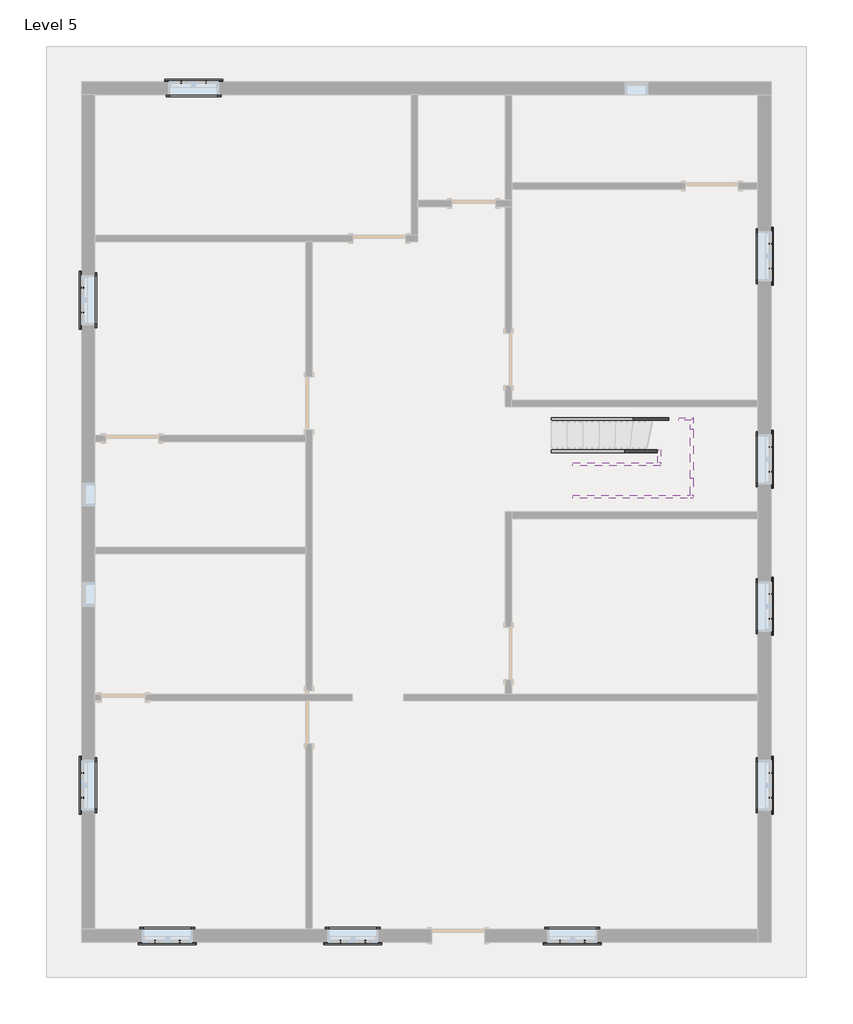
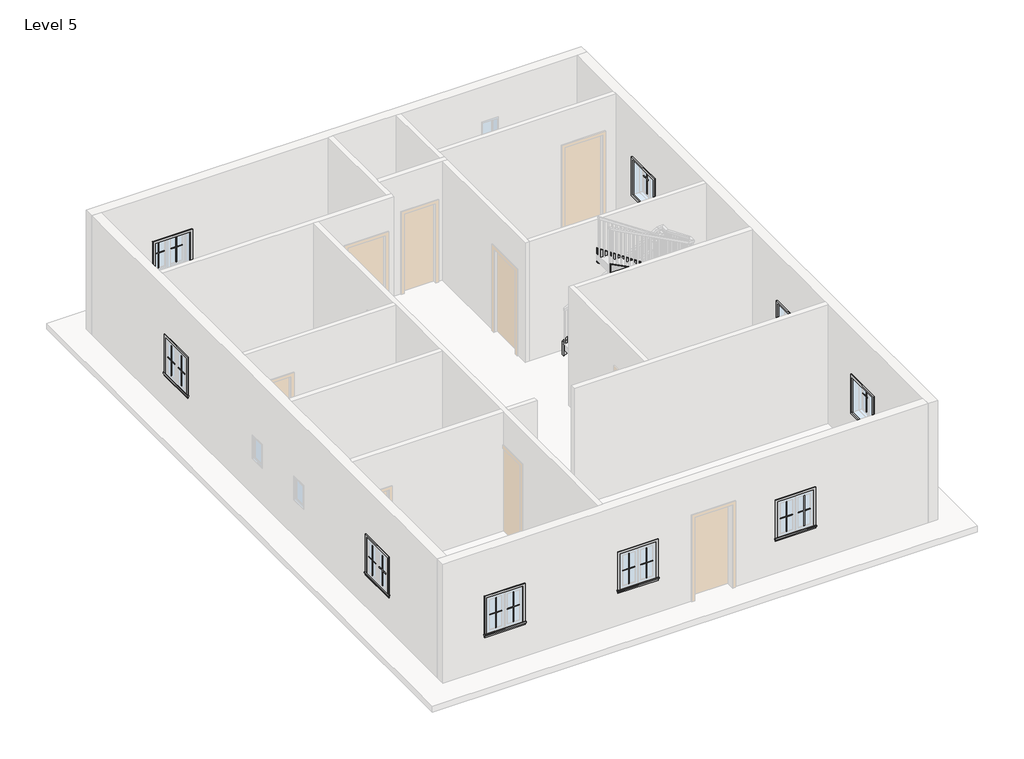
# One storey, part 3 of 3: 40 proxies, 9 members.
"""IFC4 building model written with IfcOpenShell, lengths in millimetres."""

from ifc_helpers import new_model, si_unit, frame, origin, place, context, project, spatial, polyline, outline, extrude, transform, mapped, element, save
from components import muntin_pattern_2x2_muntin_pattern_2x2_b3fe6957, muntin_pattern_2x2_muntin_pattern_2x2_3e0ecaf2, trim_window_exterior_flat_with_sill_41619996, trim_window_interior_flat_picture_frame_51c85655

model = new_model("IFC4")

# Units and contexts
model_context = context("Model", 3, world=origin())
ifc_project = project(units=[si_unit("LENGTHUNIT", "METRE", prefix="MILLI")], contexts=[model_context])

# Site, building, storey
site = spatial("IfcSite", under=ifc_project)
building = spatial("IfcBuilding", under=site)
storey = spatial("IfcBuildingStorey", under=building, Name="Level 5", Elevation=9601.2)

# Proxies
placement = place(None, origin())
muntin_pattern_2x2_muntin_pattern_2x2_shape = muntin_pattern_2x2_muntin_pattern_2x2_b3fe6957(model_context)
element("IfcBuildingElementProxy", 1, Name="Muntin Pattern_2x2 : Muntin Pattern_2x2", ObjectType="Muntin Pattern_2x2 : Muntin Pattern_2x2", at=placement, inside=storey, context=model_context, shape_type="MappedRepresentation", body=[
    mapped(muntin_pattern_2x2_muntin_pattern_2x2_shape, transform((-5581.2368007, 9072.452558, 10585.45), x_axis=(1.0, 0.0, 0.0), y_axis=(0.0, 1.0, 0.0), z_axis=(0.0, 0.0, 1.0))),
])
element("IfcBuildingElementProxy", 2, Name="Muntin Pattern_2x2 : Muntin Pattern_2x2", ObjectType="Muntin Pattern_2x2 : Muntin Pattern_2x2", at=placement, inside=storey, context=model_context, shape_type="MappedRepresentation", body=[
    mapped(muntin_pattern_2x2_muntin_pattern_2x2_shape, transform((-7300.4993007, 5076.715058, 10585.45), x_axis=(0.0, 1.0, 0.0), y_axis=(-1.0, 0.0, 0.0), z_axis=(0.0, 0.0, 1.0))),
])
element("IfcBuildingElementProxy", 3, Name="Muntin Pattern_2x2 : Muntin Pattern_2x2", ObjectType="Muntin Pattern_2x2 : Muntin Pattern_2x2", at=placement, inside=storey, context=model_context, shape_type="MappedRepresentation", body=[
    mapped(muntin_pattern_2x2_muntin_pattern_2x2_shape, transform((4643.8506993, 6267.340058, 10585.45), x_axis=(0.0, -1.0, 0.0), y_axis=(1.0, 0.0, 0.0), z_axis=(0.0, 0.0, 1.0))),
])
element("IfcBuildingElementProxy", 4, Name="Muntin Pattern_2x2 : Muntin Pattern_2x2", ObjectType="Muntin Pattern_2x2 : Muntin Pattern_2x2", at=placement, inside=storey, context=model_context, shape_type="MappedRepresentation", body=[
    mapped(muntin_pattern_2x2_muntin_pattern_2x2_shape, transform((4643.8506993, 2743.090058, 10585.45), x_axis=(0.0, -1.0, 0.0), y_axis=(1.0, 0.0, 0.0), z_axis=(0.0, 0.0, 1.0))),
])
element("IfcBuildingElementProxy", 5, Name="Muntin Pattern_2x2 : Muntin Pattern_2x2", ObjectType="Muntin Pattern_2x2 : Muntin Pattern_2x2", at=placement, inside=storey, context=model_context, shape_type="MappedRepresentation", body=[
    mapped(muntin_pattern_2x2_muntin_pattern_2x2_shape, transform((4643.8506993, 190.390058, 10585.45), x_axis=(0.0, -1.0, 0.0), y_axis=(1.0, 0.0, 0.0), z_axis=(0.0, 0.0, 1.0))),
])
element("IfcBuildingElementProxy", 6, Name="Muntin Pattern_2x2 : Muntin Pattern_2x2", ObjectType="Muntin Pattern_2x2 : Muntin Pattern_2x2", at=placement, inside=storey, context=model_context, shape_type="MappedRepresentation", body=[
    mapped(muntin_pattern_2x2_muntin_pattern_2x2_shape, transform((4643.8506993, -2914.759942, 10585.45), x_axis=(0.0, -1.0, 0.0), y_axis=(1.0, 0.0, 0.0), z_axis=(0.0, 0.0, 1.0))),
])
element("IfcBuildingElementProxy", 7, Name="Muntin Pattern_2x2 : Muntin Pattern_2x2", ObjectType="Muntin Pattern_2x2 : Muntin Pattern_2x2", at=placement, inside=storey, context=model_context, shape_type="MappedRepresentation", body=[
    mapped(muntin_pattern_2x2_muntin_pattern_2x2_shape, transform((1419.6381993, -5843.697442, 10585.45), x_axis=(-1.0, 0.0, 0.0), y_axis=(0.0, -1.0, 0.0), z_axis=(0.0, 0.0, 1.0))),
])
element("IfcBuildingElementProxy", 8, Name="Muntin Pattern_2x2 : Muntin Pattern_2x2", ObjectType="Muntin Pattern_2x2 : Muntin Pattern_2x2", at=placement, inside=storey, context=model_context, shape_type="MappedRepresentation", body=[
    mapped(muntin_pattern_2x2_muntin_pattern_2x2_shape, transform((-2390.3618007, -5843.697442, 10585.45), x_axis=(-1.0, 0.0, 0.0), y_axis=(0.0, -1.0, 0.0), z_axis=(0.0, 0.0, 1.0))),
])
element("IfcBuildingElementProxy", 9, Name="Muntin Pattern_2x2 : Muntin Pattern_2x2", ObjectType="Muntin Pattern_2x2 : Muntin Pattern_2x2", at=placement, inside=storey, context=model_context, shape_type="MappedRepresentation", body=[
    mapped(muntin_pattern_2x2_muntin_pattern_2x2_shape, transform((-5609.8118007, -5843.697442, 10585.45), x_axis=(-1.0, 0.0, 0.0), y_axis=(0.0, -1.0, 0.0), z_axis=(0.0, 0.0, 1.0))),
])
element("IfcBuildingElementProxy", 10, Name="Muntin Pattern_2x2 : Muntin Pattern_2x2", ObjectType="Muntin Pattern_2x2 : Muntin Pattern_2x2", at=placement, inside=storey, context=model_context, shape_type="MappedRepresentation", body=[
    mapped(muntin_pattern_2x2_muntin_pattern_2x2_shape, transform((-7300.4993007, -3343.384942, 10585.45), x_axis=(0.0, 1.0, 0.0), y_axis=(-1.0, 0.0, 0.0), z_axis=(0.0, 0.0, 1.0))),
])
muntin_pattern_2x2_muntin_pattern_2x2_2_shape = muntin_pattern_2x2_muntin_pattern_2x2_3e0ecaf2(model_context)
element("IfcBuildingElementProxy", 11, Name="Muntin Pattern_2x2 : Muntin Pattern_2x2", ObjectType="Muntin Pattern_2x2 : Muntin Pattern_2x2", at=placement, inside=storey, context=model_context, shape_type="MappedRepresentation", body=[
    mapped(muntin_pattern_2x2_muntin_pattern_2x2_2_shape, transform((-5152.6118007, 9072.452558, 10585.45), x_axis=(-1.0, 0.0, 0.0), y_axis=(0.0, -1.0, 0.0), z_axis=(0.0, 0.0, 1.0))),
])
element("IfcBuildingElementProxy", 12, Name="Muntin Pattern_2x2 : Muntin Pattern_2x2", ObjectType="Muntin Pattern_2x2 : Muntin Pattern_2x2", at=placement, inside=storey, context=model_context, shape_type="MappedRepresentation", body=[
    mapped(muntin_pattern_2x2_muntin_pattern_2x2_2_shape, transform((-7300.4993007, 5505.340058, 10585.45), x_axis=(0.0, -1.0, 0.0), y_axis=(1.0, 0.0, 0.0), z_axis=(0.0, 0.0, 1.0))),
])
element("IfcBuildingElementProxy", 13, Name="Muntin Pattern_2x2 : Muntin Pattern_2x2", ObjectType="Muntin Pattern_2x2 : Muntin Pattern_2x2", at=placement, inside=storey, context=model_context, shape_type="MappedRepresentation", body=[
    mapped(muntin_pattern_2x2_muntin_pattern_2x2_2_shape, transform((4643.8506993, 5838.715058, 10585.45), x_axis=(0.0, 1.0, 0.0), y_axis=(-1.0, 0.0, 0.0), z_axis=(0.0, 0.0, 1.0))),
])
element("IfcBuildingElementProxy", 14, Name="Muntin Pattern_2x2 : Muntin Pattern_2x2", ObjectType="Muntin Pattern_2x2 : Muntin Pattern_2x2", at=placement, inside=storey, context=model_context, shape_type="MappedRepresentation", body=[
    mapped(muntin_pattern_2x2_muntin_pattern_2x2_2_shape, transform((4643.8506993, 2314.465058, 10585.45), x_axis=(0.0, 1.0, 0.0), y_axis=(-1.0, 0.0, 0.0), z_axis=(0.0, 0.0, 1.0))),
])
element("IfcBuildingElementProxy", 15, Name="Muntin Pattern_2x2 : Muntin Pattern_2x2", ObjectType="Muntin Pattern_2x2 : Muntin Pattern_2x2", at=placement, inside=storey, context=model_context, shape_type="MappedRepresentation", body=[
    mapped(muntin_pattern_2x2_muntin_pattern_2x2_2_shape, transform((4643.8506993, -238.234942, 10585.45), x_axis=(0.0, 1.0, 0.0), y_axis=(-1.0, 0.0, 0.0), z_axis=(0.0, 0.0, 1.0))),
])
element("IfcBuildingElementProxy", 16, Name="Muntin Pattern_2x2 : Muntin Pattern_2x2", ObjectType="Muntin Pattern_2x2 : Muntin Pattern_2x2", at=placement, inside=storey, context=model_context, shape_type="MappedRepresentation", body=[
    mapped(muntin_pattern_2x2_muntin_pattern_2x2_2_shape, transform((4643.8506993, -3343.384942, 10585.45), x_axis=(0.0, 1.0, 0.0), y_axis=(-1.0, 0.0, 0.0), z_axis=(0.0, 0.0, 1.0))),
])
element("IfcBuildingElementProxy", 17, Name="Muntin Pattern_2x2 : Muntin Pattern_2x2", ObjectType="Muntin Pattern_2x2 : Muntin Pattern_2x2", at=placement, inside=storey, context=model_context, shape_type="MappedRepresentation", body=[
    mapped(muntin_pattern_2x2_muntin_pattern_2x2_2_shape, transform((991.0131993, -5843.697442, 10585.45), x_axis=(1.0, 0.0, 0.0), y_axis=(0.0, 1.0, 0.0), z_axis=(0.0, 0.0, 1.0))),
])
element("IfcBuildingElementProxy", 18, Name="Muntin Pattern_2x2 : Muntin Pattern_2x2", ObjectType="Muntin Pattern_2x2 : Muntin Pattern_2x2", at=placement, inside=storey, context=model_context, shape_type="MappedRepresentation", body=[
    mapped(muntin_pattern_2x2_muntin_pattern_2x2_2_shape, transform((-2818.9868007, -5843.697442, 10585.45), x_axis=(1.0, 0.0, 0.0), y_axis=(0.0, 1.0, 0.0), z_axis=(0.0, 0.0, 1.0))),
])
element("IfcBuildingElementProxy", 19, Name="Muntin Pattern_2x2 : Muntin Pattern_2x2", ObjectType="Muntin Pattern_2x2 : Muntin Pattern_2x2", at=placement, inside=storey, context=model_context, shape_type="MappedRepresentation", body=[
    mapped(muntin_pattern_2x2_muntin_pattern_2x2_2_shape, transform((-6038.4368007, -5843.697442, 10585.45), x_axis=(1.0, 0.0, 0.0), y_axis=(0.0, 1.0, 0.0), z_axis=(0.0, 0.0, 1.0))),
])
element("IfcBuildingElementProxy", 20, Name="Muntin Pattern_2x2 : Muntin Pattern_2x2", ObjectType="Muntin Pattern_2x2 : Muntin Pattern_2x2", at=placement, inside=storey, context=model_context, shape_type="MappedRepresentation", body=[
    mapped(muntin_pattern_2x2_muntin_pattern_2x2_2_shape, transform((-7300.4993007, -2914.759942, 10585.45), x_axis=(0.0, -1.0, 0.0), y_axis=(1.0, 0.0, 0.0), z_axis=(0.0, 0.0, 1.0))),
])
trim_window_exterior_flat_with_sill_shape = trim_window_exterior_flat_with_sill_41619996(model_context)
element("IfcBuildingElementProxy", 21, Name="Trim-Window-Exterior-Flat : with Sill", ObjectType="Trim-Window-Exterior-Flat : with Sill", at=placement, inside=storey, context=model_context, shape_type="MappedRepresentation", body=[
    mapped(trim_window_exterior_flat_with_sill_shape, transform((-5366.9243007, 9081.977558, 11430.0), x_axis=(-1.0, 0.0, 0.0), y_axis=(0.0, 0.0, 1.0), z_axis=(0.0, 1.0, 0.0))),
])
element("IfcBuildingElementProxy", 22, Name="Trim-Window-Exterior-Flat : with Sill", ObjectType="Trim-Window-Exterior-Flat : with Sill", at=placement, inside=storey, context=model_context, shape_type="MappedRepresentation", body=[
    mapped(trim_window_exterior_flat_with_sill_shape, transform((-7310.0243007, 5291.027558, 11430.0), x_axis=(0.0, -1.0, 0.0), y_axis=(0.0, 0.0, 1.0), z_axis=(-1.0, 0.0, 0.0))),
])
element("IfcBuildingElementProxy", 23, Name="Trim-Window-Exterior-Flat : with Sill", ObjectType="Trim-Window-Exterior-Flat : with Sill", at=placement, inside=storey, context=model_context, shape_type="MappedRepresentation", body=[
    mapped(trim_window_exterior_flat_with_sill_shape, transform((4653.3756993, 6053.027558, 11430.0), x_axis=(0.0, 1.0, 0.0), y_axis=(0.0, 0.0, 1.0), z_axis=(1.0, 0.0, 0.0))),
])
element("IfcBuildingElementProxy", 24, Name="Trim-Window-Exterior-Flat : with Sill", ObjectType="Trim-Window-Exterior-Flat : with Sill", at=placement, inside=storey, context=model_context, shape_type="MappedRepresentation", body=[
    mapped(trim_window_exterior_flat_with_sill_shape, transform((4653.3756993, 2528.777558, 11430.0), x_axis=(0.0, 1.0, 0.0), y_axis=(0.0, 0.0, 1.0), z_axis=(1.0, 0.0, 0.0))),
])
element("IfcBuildingElementProxy", 25, Name="Trim-Window-Exterior-Flat : with Sill", ObjectType="Trim-Window-Exterior-Flat : with Sill", at=placement, inside=storey, context=model_context, shape_type="MappedRepresentation", body=[
    mapped(trim_window_exterior_flat_with_sill_shape, transform((4653.3756993, -23.922442, 11430.0), x_axis=(0.0, 1.0, 0.0), y_axis=(0.0, 0.0, 1.0), z_axis=(1.0, 0.0, 0.0))),
])
element("IfcBuildingElementProxy", 26, Name="Trim-Window-Exterior-Flat : with Sill", ObjectType="Trim-Window-Exterior-Flat : with Sill", at=placement, inside=storey, context=model_context, shape_type="MappedRepresentation", body=[
    mapped(trim_window_exterior_flat_with_sill_shape, transform((4653.3756993, -3129.072442, 11430.0), x_axis=(0.0, 1.0, 0.0), y_axis=(0.0, 0.0, 1.0), z_axis=(1.0, 0.0, 0.0))),
])
element("IfcBuildingElementProxy", 27, Name="Trim-Window-Exterior-Flat : with Sill", ObjectType="Trim-Window-Exterior-Flat : with Sill", at=placement, inside=storey, context=model_context, shape_type="MappedRepresentation", body=[
    mapped(trim_window_exterior_flat_with_sill_shape, transform((1205.3256993, -5853.222442, 11430.0), x_axis=(1.0, 0.0, 0.0), y_axis=(0.0, 0.0, 1.0), z_axis=(0.0, -1.0, 0.0))),
])
element("IfcBuildingElementProxy", 28, Name="Trim-Window-Exterior-Flat : with Sill", ObjectType="Trim-Window-Exterior-Flat : with Sill", at=placement, inside=storey, context=model_context, shape_type="MappedRepresentation", body=[
    mapped(trim_window_exterior_flat_with_sill_shape, transform((-2604.6743007, -5853.222442, 11430.0), x_axis=(1.0, 0.0, 0.0), y_axis=(0.0, 0.0, 1.0), z_axis=(0.0, -1.0, 0.0))),
])
element("IfcBuildingElementProxy", 29, Name="Trim-Window-Exterior-Flat : with Sill", ObjectType="Trim-Window-Exterior-Flat : with Sill", at=placement, inside=storey, context=model_context, shape_type="MappedRepresentation", body=[
    mapped(trim_window_exterior_flat_with_sill_shape, transform((-5824.1243007, -5853.222442, 11430.0), x_axis=(1.0, 0.0, 0.0), y_axis=(0.0, 0.0, 1.0), z_axis=(0.0, -1.0, 0.0))),
])
element("IfcBuildingElementProxy", 30, Name="Trim-Window-Exterior-Flat : with Sill", ObjectType="Trim-Window-Exterior-Flat : with Sill", at=placement, inside=storey, context=model_context, shape_type="MappedRepresentation", body=[
    mapped(trim_window_exterior_flat_with_sill_shape, transform((-7310.0243007, -3129.072442, 11430.0), x_axis=(0.0, -1.0, 0.0), y_axis=(0.0, 0.0, 1.0), z_axis=(-1.0, 0.0, 0.0))),
])
trim_window_interior_flat_picture_frame_shape = trim_window_interior_flat_picture_frame_51c85655(model_context)
element("IfcBuildingElementProxy", 31, Name="Trim-Window-Interior-Flat : Picture Frame", ObjectType="Trim-Window-Interior-Flat : Picture Frame", at=placement, inside=storey, context=model_context, shape_type="MappedRepresentation", body=[
    mapped(trim_window_interior_flat_picture_frame_shape, transform((-5366.9243007, 8853.377558, 11430.0), x_axis=(1.0, 0.0, 0.0), y_axis=(0.0, 0.0, 1.0), z_axis=(0.0, -1.0, 0.0))),
])
element("IfcBuildingElementProxy", 32, Name="Trim-Window-Interior-Flat : Picture Frame", ObjectType="Trim-Window-Interior-Flat : Picture Frame", at=placement, inside=storey, context=model_context, shape_type="MappedRepresentation", body=[
    mapped(trim_window_interior_flat_picture_frame_shape, transform((-7081.4243007, 5291.027558, 11430.0), x_axis=(0.0, 1.0, 0.0), y_axis=(0.0, 0.0, 1.0), z_axis=(1.0, 0.0, 0.0))),
])
element("IfcBuildingElementProxy", 33, Name="Trim-Window-Interior-Flat : Picture Frame", ObjectType="Trim-Window-Interior-Flat : Picture Frame", at=placement, inside=storey, context=model_context, shape_type="MappedRepresentation", body=[
    mapped(trim_window_interior_flat_picture_frame_shape, transform((4424.7756993, 6053.027558, 11430.0), x_axis=(0.0, -1.0, 0.0), y_axis=(0.0, 0.0, 1.0), z_axis=(-1.0, 0.0, 0.0))),
])
element("IfcBuildingElementProxy", 34, Name="Trim-Window-Interior-Flat : Picture Frame", ObjectType="Trim-Window-Interior-Flat : Picture Frame", at=placement, inside=storey, context=model_context, shape_type="MappedRepresentation", body=[
    mapped(trim_window_interior_flat_picture_frame_shape, transform((4424.7756993, 2528.777558, 11430.0), x_axis=(0.0, -1.0, 0.0), y_axis=(0.0, 0.0, 1.0), z_axis=(-1.0, 0.0, 0.0))),
])
element("IfcBuildingElementProxy", 35, Name="Trim-Window-Interior-Flat : Picture Frame", ObjectType="Trim-Window-Interior-Flat : Picture Frame", at=placement, inside=storey, context=model_context, shape_type="MappedRepresentation", body=[
    mapped(trim_window_interior_flat_picture_frame_shape, transform((4424.7756993, -23.922442, 11430.0), x_axis=(0.0, -1.0, 0.0), y_axis=(0.0, 0.0, 1.0), z_axis=(-1.0, 0.0, 0.0))),
])
element("IfcBuildingElementProxy", 36, Name="Trim-Window-Interior-Flat : Picture Frame", ObjectType="Trim-Window-Interior-Flat : Picture Frame", at=placement, inside=storey, context=model_context, shape_type="MappedRepresentation", body=[
    mapped(trim_window_interior_flat_picture_frame_shape, transform((4424.7756993, -3129.072442, 11430.0), x_axis=(0.0, -1.0, 0.0), y_axis=(0.0, 0.0, 1.0), z_axis=(-1.0, 0.0, 0.0))),
])
element("IfcBuildingElementProxy", 37, Name="Trim-Window-Interior-Flat : Picture Frame", ObjectType="Trim-Window-Interior-Flat : Picture Frame", at=placement, inside=storey, context=model_context, shape_type="MappedRepresentation", body=[
    mapped(trim_window_interior_flat_picture_frame_shape, transform((1205.3256993, -5624.622442, 11430.0), x_axis=(-1.0, 0.0, 0.0), y_axis=(0.0, 0.0, 1.0), z_axis=(0.0, 1.0, 0.0))),
])
element("IfcBuildingElementProxy", 38, Name="Trim-Window-Interior-Flat : Picture Frame", ObjectType="Trim-Window-Interior-Flat : Picture Frame", at=placement, inside=storey, context=model_context, shape_type="MappedRepresentation", body=[
    mapped(trim_window_interior_flat_picture_frame_shape, transform((-2604.6743007, -5624.622442, 11430.0), x_axis=(-1.0, 0.0, 0.0), y_axis=(0.0, 0.0, 1.0), z_axis=(0.0, 1.0, 0.0))),
])
element("IfcBuildingElementProxy", 39, Name="Trim-Window-Interior-Flat : Picture Frame", ObjectType="Trim-Window-Interior-Flat : Picture Frame", at=placement, inside=storey, context=model_context, shape_type="MappedRepresentation", body=[
    mapped(trim_window_interior_flat_picture_frame_shape, transform((-5824.1243007, -5624.622442, 11430.0), x_axis=(-1.0, 0.0, 0.0), y_axis=(0.0, 0.0, 1.0), z_axis=(0.0, 1.0, 0.0))),
])
element("IfcBuildingElementProxy", 40, Name="Trim-Window-Interior-Flat : Picture Frame", ObjectType="Trim-Window-Interior-Flat : Picture Frame", at=placement, inside=storey, context=model_context, shape_type="MappedRepresentation", body=[
    mapped(trim_window_interior_flat_picture_frame_shape, transform((-7081.4243007, -3129.072442, 11430.0), x_axis=(0.0, 1.0, 0.0), y_axis=(0.0, 0.0, 1.0), z_axis=(1.0, 0.0, 0.0))),
])

# Members
element("IfcMember", 41, ObjectType="Stringer - 2\" Width", at=placement, inside=storey, context=model_context, shape_type="SweptSolid", body=[
    extrude(outline(polyline([(9989.6746569, 838.4202681), (9639.0072902, 838.4202681), (10898.6160324, 3052.6525996), (11249.2833991, 3052.6525996), (9989.6746569, 838.4202681)])), frame((0.0, 3202.4524989, 0.0), z_axis=(0.0, 1.0, 0.0), x_axis=(0.0, 0.0, 1.0)), (0.0, 0.0, 1.0), 50.8),
])
element("IfcMember", 42, ObjectType="Stringer - 2\" Width", at=placement, inside=storey, context=model_context, shape_type="SweptSolid", body=[
    extrude(outline(polyline([(3052.6525996, 3202.4524989), (3052.6525996, 3253.2524989), (3298.782332, 3253.2524989), (3247.982332, 3202.4524989), (3052.6525996, 3202.4524989)])), frame((0.0, 0.0, 10898.6160324), z_axis=(0.0, 0.0, 1.0), x_axis=(1.0, 0.0, 0.0)), (0.0, 0.0, 1.0), 350.6673667),
])
element("IfcMember", 43, ObjectType="Stringer - 2\" Width", at=placement, inside=storey, context=model_context, shape_type="SweptSolid", body=[
    extrude(outline(polyline([(3247.982332, 3202.4524989), (3298.782332, 3253.2524989), (3298.782332, 3048.1586437), (3247.982332, 3048.1586437), (3247.982332, 3202.4524989)])), frame((0.0, 0.0, 10898.6160324), z_axis=(0.0, 0.0, 1.0), x_axis=(1.0, 0.0, 0.0)), (0.0, 0.0, 1.0), 350.6673667),
])
element("IfcMember", 44, ObjectType="Stringer - 2\" Width", at=placement, inside=storey, context=model_context, shape_type="SweptSolid", body=[
    extrude(outline(polyline([(3048.1586437, 11249.2833991), (3048.1586437, 10898.6160324), (2198.376501, 11254.1779505), (2198.376501, 11604.8453172), (3048.1586437, 11249.2833991)])), frame((3247.982332, 0.0, 0.0), z_axis=(1.0, 0.0, 0.0), x_axis=(0.0, 1.0, 0.0)), (0.0, 0.0, 1.0), 50.8),
])
element("IfcMember", 45, ObjectType="Stringer - 2\" Width", at=placement, inside=storey, context=model_context, shape_type="SweptSolid", body=[
    extrude(outline(polyline([(3247.982332, 2198.376501), (3298.782332, 2198.376501), (3298.782332, 1905.9026171), (3247.982332, 1905.9026171), (3247.982332, 2198.376501)])), frame((0.0, 0.0, 11263.1761112), z_axis=(0.0, 0.0, 1.0), x_axis=(1.0, 0.0, 0.0)), (0.0, 0.0, 1.0), 330.4053693),
])
element("IfcMember", 46, ObjectType="Stringer - 2\" Width", at=placement, inside=storey, context=model_context, shape_type="SweptSolid", body=[
    extrude(outline(polyline([(9975.2558321, 838.4202681), (9612.3163437, 838.4202681), (10808.3401496, 2688.6073911), (11171.2796379, 2688.6073911), (9975.2558321, 838.4202681)])), frame((0.0, 2643.077558, 0.0), z_axis=(0.0, 1.0, 0.0), x_axis=(0.0, 0.0, 1.0)), (0.0, 0.0, 1.0), 50.8),
])
element("IfcMember", 47, ObjectType="Stringer - 2\" Width", at=placement, inside=storey, context=model_context, shape_type="SweptSolid", body=[
    extrude(outline(polyline([(2693.877558, 11338.6149577), (2693.877558, 10891.3996268), (2465.277558, 11136.8439445), (2465.277558, 11584.0592754), (2693.877558, 11338.6149577)])), frame((2688.6073911, 0.0, 0.0), z_axis=(1.0, 0.0, 0.0), x_axis=(0.0, 1.0, 0.0)), (0.0, 0.0, 1.0), 50.8),
])
element("IfcMember", 48, ObjectType="Stringer - 2\" Width", at=placement, inside=storey, context=model_context, shape_type="SweptSolid", body=[
    extrude(outline(polyline([(11301.9150039, 2739.4073911), (11671.891358, 2739.4073911), (12723.0229383, 1211.6756993), (12353.0465842, 1211.6756993), (11301.9150039, 2739.4073911)])), frame((0.0, 2414.477558, 0.0), z_axis=(0.0, 1.0, 0.0), x_axis=(0.0, 0.0, 1.0)), (0.0, 0.0, 1.0), 50.8),
])
element("IfcMember", 49, ObjectType="Stringer - 2\" Width", at=placement, inside=storey, context=model_context, shape_type="SweptSolid", body=[
    extrude(outline(polyline([(11288.7814805, 3298.782332), (11567.1410006, 3298.782332), (12653.442202, 1211.6756993), (12323.0368327, 1211.6756993), (11288.7814805, 3198.7868271), (11288.7814805, 3298.782332)])), frame((0.0, 1855.1026171, 0.0), z_axis=(0.0, 1.0, 0.0), x_axis=(0.0, 0.0, 1.0)), (0.0, 0.0, 1.0), 50.8),
])

save(model, "model.ifc")

# Revit data of these elements
# Type "Muntin Pattern_2x2 : Muntin Pattern_2x2"
#   Width [instance default] = 4' - 0"
#   Thickness = 0' - 0 1/2"
#   Height [instance default] = 4' - 0"
#   Distance = 0' - 0 3/4"
#   Interior Material [instance default] = none
#   Exterior Material [instance default] = none
#   Default Elevation = 0
# Type "Trim-Window-Exterior-Flat : with Sill"
#   Trim Width = 0' - 2 1/4"
#   Trim Thickness_Picture Frame = 0' - 1 1/4"
#   Trim Thickness_with Sill = 0' - 0 3/4"
#   Sill Thickness = 0' - 1 1/4"
#   Opening Width [instance default] = 2' - 0"
#   Opening Height [instance default] = 3' - 0"
#   Default Elevation = 4' - 0"
#   Sill = yes
#   Picture Frame = no
#   Trim Material [instance default] = none
# Type "Trim-Window-Interior-Flat : Picture Frame"
#   Trim Thickness_Picture Frame = 0' - 1 1/4"
#   Trim Width = 0' - 2 1/4"
#   Trim Thickness_with Sill = 0' - 0 3/4"
#   Sill Thickness = 0' - 1 1/4"
#   Opening Width [instance default] = 2' - 0"
#   Opening Height [instance default] = 3' - 0"
#   Default Elevation = 4' - 0"
#   Sill = no
#   Picture Frame = yes
#   Trim Material [instance default] = none
# Elements 1, 2, 3, 4, 5, 6, 7, 8, 9, 10, 11, 12, 13, 14, 15, 16, 17, 18, 19, 20 (IfcBuildingElementProxy, "Muntin Pattern_2x2 : Muntin Pattern_2x2")
#   Width = 0' - 11 5/8"
#   Height = 2' - 6 1/2"
#   Interior Material = Wood - Stained
#   Exterior Material = Clad - White
#   Phase Created = New Construction
#   Materials on its faces: "Clad - White", "Wood - Stained"
# Elements 21, 22, 23, 24, 25, 26, 27, 28, 29, 30 (IfcBuildingElementProxy, "Trim-Window-Exterior-Flat : with Sill")
#   Opening Width = 2' - 10"
#   Opening Height = 3' - 0"
#   Trim Material = Clad - White
#   Phase Created = New Construction
#   Materials on its faces: "Clad - White"
# Elements 31, 32, 33, 34, 35, 36, 37, 38, 39, 40 (IfcBuildingElementProxy, "Trim-Window-Interior-Flat : Picture Frame")
#   Opening Width = 2' - 10"
#   Opening Height = 3' - 0"
#   Trim Material = Wood - Stained
#   Phase Created = New Construction
#   Materials on its faces: "Wood - Stained"
# Elements 41, 42, 43, 44, 45, 46, 47, 48, 49 (IfcMember, "Stringer - 2\" Width")
#   Phase Created = New Construction
# Materials
#   "Clad - White": class "Wood", colour RGB 242 242 238, transparency 0, Cost = 0
#   "Wood - Stained": class "Wood", colour RGB 224 178 126, transparency 0, Cost = 0
